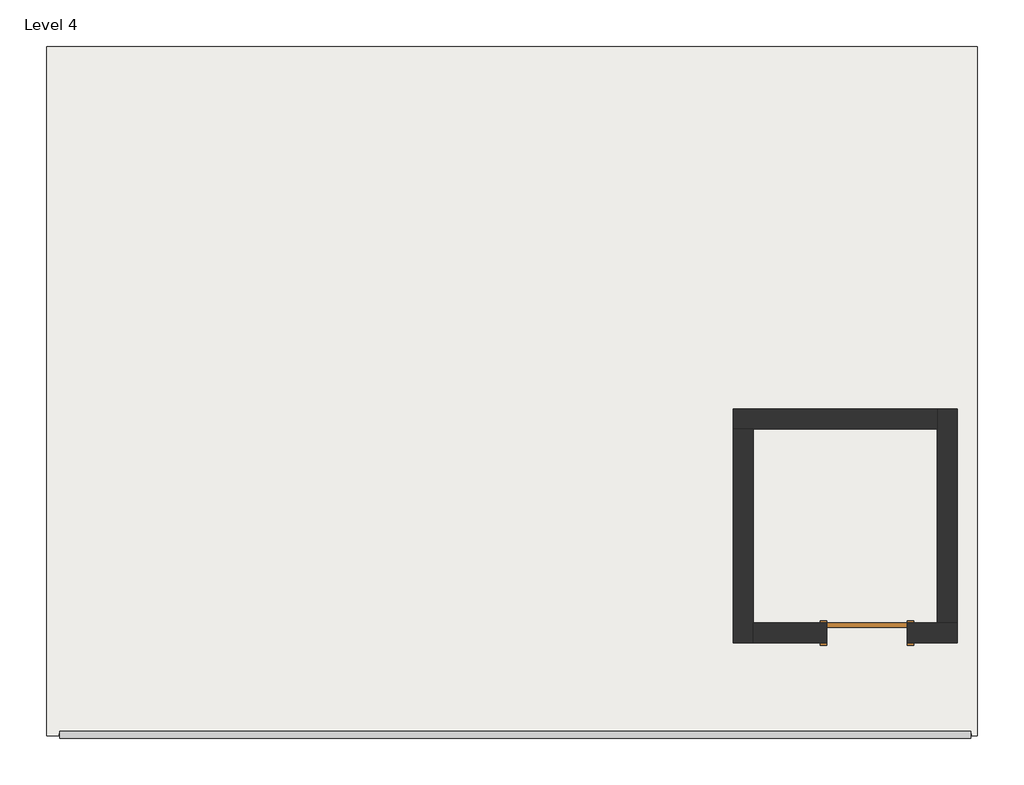
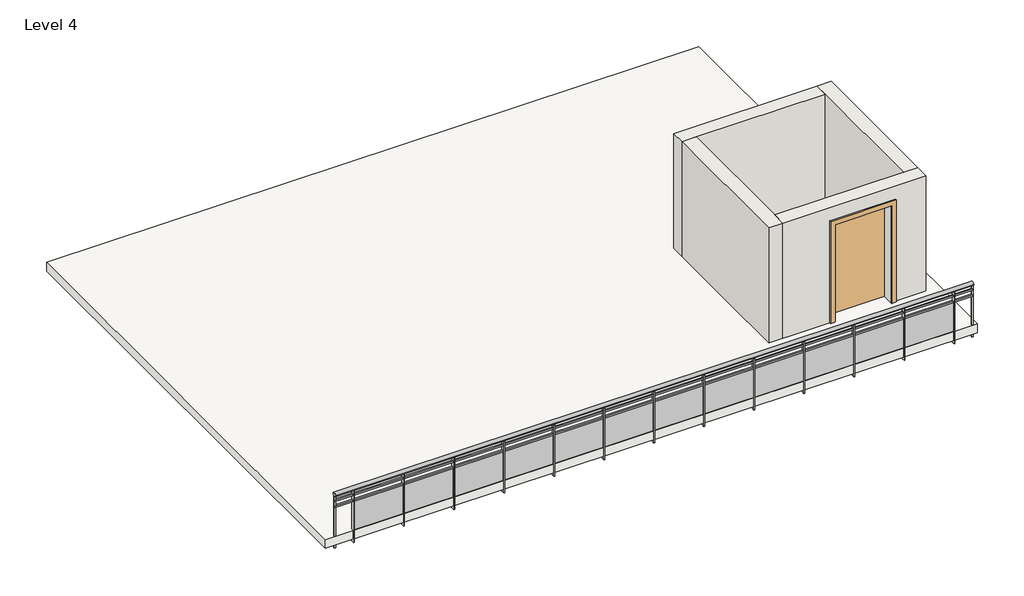
# One storey: 4 walls, 1 door, 1 railing, 1 roof.
"""IFC4 building model written with IfcOpenShell, lengths in millimetres."""

from ifc_helpers import new_model, si_unit, point, frame, origin, place, context, project, spatial, polyline, ellipse_curve, trimmed, outline, extrude, faceted_brep, transform, mapped, element, save
from ifc_brep_helpers import plane_surface, extruded_surface, advanced_brep
from components import door_0ca8825f

model = new_model("IFC4")

# Units and contexts
model_context = context("Model", 3, world=origin())
ifc_project = project(units=[si_unit("LENGTHUNIT", "METRE", prefix="MILLI")], contexts=[model_context])

# Site, building, storey
site = spatial("IfcSite", under=ifc_project)
building = spatial("IfcBuilding", under=site)
storey = spatial("IfcBuildingStorey", under=building, Name="Level 4", Elevation=6248.4)

# Door
placement = place(None, origin())
door_shape = door_0ca8825f(model_context)
element("IfcDoor", 1, ObjectType="Single-Flush : 36\" x 84\"", at=placement, inside=storey, context=model_context, shape_type="MappedRepresentation", body=[
    mapped(door_shape, transform((-524.0379854, -4635.5538577, 6248.4), x_axis=(1.0, 0.0, 0.0), y_axis=(0.0, 1.0, 0.0), z_axis=(0.0, 0.0, 1.0))),
])

# Railing
element("IfcRailing", 2, ObjectType="Glass Panel - Bottom Fill", at=placement, inside=storey, context=model_context, shape_type="SolidModel", body=[
    advanced_brep(
    [(657.0620146, -5831.8506821, 7416.8), (657.0620146, -5755.6506821, 7416.8), (-9706.1379854, -5831.8506821, 7416.8), (-9706.1379854, -5755.6506821, 7416.8)],
    [
        (0, 1, ellipse_curve(frame((657.0620146, -5793.7506821, 7416.8), z_axis=(1.0, 0.0, 0.0), x_axis=(0.0, 1.0, 0.0)), 38.1, 28.575)),
        (1, 0, ellipse_curve(frame((657.0620146, -5793.7506821, 7416.8), z_axis=(1.0, 0.0, 0.0), x_axis=(0.0, 1.0, 0.0)), 38.1, 28.575)),
        (2, 3, ellipse_curve(frame((-9706.1379854, -5793.7506821, 7416.8), z_axis=(-1.0, 0.0, 0.0), x_axis=(0.0, 1.0, 0.0)), 38.1, 28.575)),
        (3, 2, ellipse_curve(frame((-9706.1379854, -5793.7506821, 7416.8), z_axis=(-1.0, 0.0, 0.0), x_axis=(0.0, 1.0, 0.0)), 38.1, 28.575)),
        (0, 2),
        (3, 1),
    ],
    [
        plane_surface(frame((657.0620146, -5793.7506821, 7416.8), z_axis=(1.0, 0.0, 0.0), x_axis=(0.0, -1.0, 0.0))),
        plane_surface(frame((-9706.1379854, -5793.7506821, 7416.8), z_axis=(-1.0, 0.0, 0.0), x_axis=(0.0, -1.0, 0.0))),
        extruded_surface(trimmed(ellipse_curve(frame((-9706.1379854, -5793.7506821, 7416.8), z_axis=(1.0, 0.0, 0.0), x_axis=(0.0, 1.0, 0.0)), 38.1, 28.575), [point((-9706.1379854, -5831.8506821, 7416.8))], [point((-9706.1379854, -5755.6506821, 7416.8))], True, "CARTESIAN"), (10363.2, 0.0, 0.0), 10363.2),
        extruded_surface(trimmed(ellipse_curve(frame((-9706.1379854, -5793.7506821, 7416.8), z_axis=(1.0, 0.0, 0.0), x_axis=(0.0, 1.0, 0.0)), 38.1, 28.575), [point((-9706.1379854, -5755.6506821, 7416.8))], [point((-9706.1379854, -5831.8506821, 7416.8))], True, "CARTESIAN"), (10363.2, 0.0, 0.0), 10363.2),
    ],
    [
        (0, [[1, 2]]),
        (1, [[3, 4]]),
        (2, [[-1, 5, -4, 6]]),
        (3, [[-2, -6, -3, -5]]),
    ],
),
    extrude(outline(polyline([(657.0620146, -5781.0506821), (657.0620146, -5806.4506821), (-9706.1379854, -5806.4506821), (-9706.1379854, -5781.0506821), (657.0620146, -5781.0506821)])), frame((0.0, 0.0, 7302.5), z_axis=(0.0, 0.0, 1.0), x_axis=(1.0, 0.0, 0.0)), (0.0, 0.0, 1.0), 25.4),
    extrude(outline(polyline([(657.0620146, -5781.0506821), (657.0620146, -5806.4506821), (-9706.1379854, -5806.4506821), (-9706.1379854, -5781.0506821), (657.0620146, -5781.0506821)])), frame((0.0, 0.0, 7200.9), z_axis=(0.0, 0.0, 1.0), x_axis=(1.0, 0.0, 0.0)), (0.0, 0.0, 1.0), 25.4),
    extrude(outline(polyline([(-9394.9879854, -5768.3506821), (-9394.9879854, -5819.1506821), (-9407.6879854, -5819.1506821), (-9407.6879854, -5768.3506821), (-9394.9879854, -5768.3506821)])), frame((0.0, 0.0, 6502.4), z_axis=(0.0, 0.0, 1.0), x_axis=(1.0, 0.0, 0.0)), (0.0, 0.0, 1.0), 885.825),
    extrude(outline(polyline([(-8588.5379854, -5800.2858391), (-9401.3379854, -5800.2858391), (-9401.3379854, -5793.9358391), (-8588.5379854, -5793.9358391), (-8588.5379854, -5800.2858391)])), frame((0.0, 0.0, 6604.0), z_axis=(0.0, 0.0, 1.0), x_axis=(1.0, 0.0, 0.0)), (0.0, 0.0, 1.0), 596.9),
    extrude(outline(polyline([(-8582.1879854, -5768.3506821), (-8582.1879854, -5819.1506821), (-8594.8879854, -5819.1506821), (-8594.8879854, -5768.3506821), (-8582.1879854, -5768.3506821)])), frame((0.0, 0.0, 6502.4), z_axis=(0.0, 0.0, 1.0), x_axis=(1.0, 0.0, 0.0)), (0.0, 0.0, 1.0), 885.825),
    extrude(outline(polyline([(-7775.7379854, -5800.2858391), (-8588.5379854, -5800.2858391), (-8588.5379854, -5793.9358391), (-7775.7379854, -5793.9358391), (-7775.7379854, -5800.2858391)])), frame((0.0, 0.0, 6604.0), z_axis=(0.0, 0.0, 1.0), x_axis=(1.0, 0.0, 0.0)), (0.0, 0.0, 1.0), 596.9),
    extrude(outline(polyline([(-7769.3879854, -5768.3506821), (-7769.3879854, -5819.1506821), (-7782.0879854, -5819.1506821), (-7782.0879854, -5768.3506821), (-7769.3879854, -5768.3506821)])), frame((0.0, 0.0, 6502.4), z_axis=(0.0, 0.0, 1.0), x_axis=(1.0, 0.0, 0.0)), (0.0, 0.0, 1.0), 885.825),
    extrude(outline(polyline([(-6962.9379854, -5800.2858391), (-7775.7379854, -5800.2858391), (-7775.7379854, -5793.9358391), (-6962.9379854, -5793.9358391), (-6962.9379854, -5800.2858391)])), frame((0.0, 0.0, 6604.0), z_axis=(0.0, 0.0, 1.0), x_axis=(1.0, 0.0, 0.0)), (0.0, 0.0, 1.0), 596.9),
    extrude(outline(polyline([(-6956.5879854, -5768.3506821), (-6956.5879854, -5819.1506821), (-6969.2879854, -5819.1506821), (-6969.2879854, -5768.3506821), (-6956.5879854, -5768.3506821)])), frame((0.0, 0.0, 6502.4), z_axis=(0.0, 0.0, 1.0), x_axis=(1.0, 0.0, 0.0)), (0.0, 0.0, 1.0), 885.825),
    extrude(outline(polyline([(-6150.1379854, -5800.2858391), (-6962.9379854, -5800.2858391), (-6962.9379854, -5793.9358391), (-6150.1379854, -5793.9358391), (-6150.1379854, -5800.2858391)])), frame((0.0, 0.0, 6604.0), z_axis=(0.0, 0.0, 1.0), x_axis=(1.0, 0.0, 0.0)), (0.0, 0.0, 1.0), 596.9),
    extrude(outline(polyline([(-6143.7879854, -5768.3506821), (-6143.7879854, -5819.1506821), (-6156.4879854, -5819.1506821), (-6156.4879854, -5768.3506821), (-6143.7879854, -5768.3506821)])), frame((0.0, 0.0, 6502.4), z_axis=(0.0, 0.0, 1.0), x_axis=(1.0, 0.0, 0.0)), (0.0, 0.0, 1.0), 885.825),
    extrude(outline(polyline([(-5337.3379854, -5800.2858391), (-6150.1379854, -5800.2858391), (-6150.1379854, -5793.9358391), (-5337.3379854, -5793.9358391), (-5337.3379854, -5800.2858391)])), frame((0.0, 0.0, 6604.0), z_axis=(0.0, 0.0, 1.0), x_axis=(1.0, 0.0, 0.0)), (0.0, 0.0, 1.0), 596.9),
    extrude(outline(polyline([(-5330.9879854, -5768.3506821), (-5330.9879854, -5819.1506821), (-5343.6879854, -5819.1506821), (-5343.6879854, -5768.3506821), (-5330.9879854, -5768.3506821)])), frame((0.0, 0.0, 6502.4), z_axis=(0.0, 0.0, 1.0), x_axis=(1.0, 0.0, 0.0)), (0.0, 0.0, 1.0), 885.825),
    extrude(outline(polyline([(-4524.5379854, -5800.2858391), (-5337.3379854, -5800.2858391), (-5337.3379854, -5793.9358391), (-4524.5379854, -5793.9358391), (-4524.5379854, -5800.2858391)])), frame((0.0, 0.0, 6604.0), z_axis=(0.0, 0.0, 1.0), x_axis=(1.0, 0.0, 0.0)), (0.0, 0.0, 1.0), 596.9),
    extrude(outline(polyline([(-4518.1879854, -5768.3506821), (-4518.1879854, -5819.1506821), (-4530.8879854, -5819.1506821), (-4530.8879854, -5768.3506821), (-4518.1879854, -5768.3506821)])), frame((0.0, 0.0, 6502.4), z_axis=(0.0, 0.0, 1.0), x_axis=(1.0, 0.0, 0.0)), (0.0, 0.0, 1.0), 885.825),
    extrude(outline(polyline([(-3711.7379854, -5800.2858391), (-4524.5379854, -5800.2858391), (-4524.5379854, -5793.9358391), (-3711.7379854, -5793.9358391), (-3711.7379854, -5800.2858391)])), frame((0.0, 0.0, 6604.0), z_axis=(0.0, 0.0, 1.0), x_axis=(1.0, 0.0, 0.0)), (0.0, 0.0, 1.0), 596.9),
    extrude(outline(polyline([(-3705.3879854, -5768.3506821), (-3705.3879854, -5819.1506821), (-3718.0879854, -5819.1506821), (-3718.0879854, -5768.3506821), (-3705.3879854, -5768.3506821)])), frame((0.0, 0.0, 6502.4), z_axis=(0.0, 0.0, 1.0), x_axis=(1.0, 0.0, 0.0)), (0.0, 0.0, 1.0), 885.825),
    extrude(outline(polyline([(-2898.9379854, -5800.2858391), (-3711.7379854, -5800.2858391), (-3711.7379854, -5793.9358391), (-2898.9379854, -5793.9358391), (-2898.9379854, -5800.2858391)])), frame((0.0, 0.0, 6604.0), z_axis=(0.0, 0.0, 1.0), x_axis=(1.0, 0.0, 0.0)), (0.0, 0.0, 1.0), 596.9),
    extrude(outline(polyline([(-2892.5879854, -5768.3506821), (-2892.5879854, -5819.1506821), (-2905.2879854, -5819.1506821), (-2905.2879854, -5768.3506821), (-2892.5879854, -5768.3506821)])), frame((0.0, 0.0, 6502.4), z_axis=(0.0, 0.0, 1.0), x_axis=(1.0, 0.0, 0.0)), (0.0, 0.0, 1.0), 885.825),
    extrude(outline(polyline([(-2086.1379854, -5800.2858391), (-2898.9379854, -5800.2858391), (-2898.9379854, -5793.9358391), (-2086.1379854, -5793.9358391), (-2086.1379854, -5800.2858391)])), frame((0.0, 0.0, 6604.0), z_axis=(0.0, 0.0, 1.0), x_axis=(1.0, 0.0, 0.0)), (0.0, 0.0, 1.0), 596.9),
    extrude(outline(polyline([(-2079.7879854, -5768.3506821), (-2079.7879854, -5819.1506821), (-2092.4879854, -5819.1506821), (-2092.4879854, -5768.3506821), (-2079.7879854, -5768.3506821)])), frame((0.0, 0.0, 6502.4), z_axis=(0.0, 0.0, 1.0), x_axis=(1.0, 0.0, 0.0)), (0.0, 0.0, 1.0), 885.825),
    extrude(outline(polyline([(-1273.3379854, -5800.2858391), (-2086.1379854, -5800.2858391), (-2086.1379854, -5793.9358391), (-1273.3379854, -5793.9358391), (-1273.3379854, -5800.2858391)])), frame((0.0, 0.0, 6604.0), z_axis=(0.0, 0.0, 1.0), x_axis=(1.0, 0.0, 0.0)), (0.0, 0.0, 1.0), 596.9),
    extrude(outline(polyline([(-1266.9879854, -5768.3506821), (-1266.9879854, -5819.1506821), (-1279.6879854, -5819.1506821), (-1279.6879854, -5768.3506821), (-1266.9879854, -5768.3506821)])), frame((0.0, 0.0, 6502.4), z_axis=(0.0, 0.0, 1.0), x_axis=(1.0, 0.0, 0.0)), (0.0, 0.0, 1.0), 885.825),
    extrude(outline(polyline([(-460.5379854, -5800.2858391), (-1273.3379854, -5800.2858391), (-1273.3379854, -5793.9358391), (-460.5379854, -5793.9358391), (-460.5379854, -5800.2858391)])), frame((0.0, 0.0, 6604.0), z_axis=(0.0, 0.0, 1.0), x_axis=(1.0, 0.0, 0.0)), (0.0, 0.0, 1.0), 596.9),
    extrude(outline(polyline([(-454.1879854, -5768.3506821), (-454.1879854, -5819.1506821), (-466.8879854, -5819.1506821), (-466.8879854, -5768.3506821), (-454.1879854, -5768.3506821)])), frame((0.0, 0.0, 6502.4), z_axis=(0.0, 0.0, 1.0), x_axis=(1.0, 0.0, 0.0)), (0.0, 0.0, 1.0), 885.825),
    extrude(outline(polyline([(352.2620146, -5800.2858391), (-460.5379854, -5800.2858391), (-460.5379854, -5793.9358391), (352.2620146, -5793.9358391), (352.2620146, -5800.2858391)])), frame((0.0, 0.0, 6604.0), z_axis=(0.0, 0.0, 1.0), x_axis=(1.0, 0.0, 0.0)), (0.0, 0.0, 1.0), 596.9),
    extrude(outline(polyline([(358.6120146, -5768.3506821), (358.6120146, -5819.1506821), (345.9120146, -5819.1506821), (345.9120146, -5768.3506821), (358.6120146, -5768.3506821)])), frame((0.0, 0.0, 6502.4), z_axis=(0.0, 0.0, 1.0), x_axis=(1.0, 0.0, 0.0)), (0.0, 0.0, 1.0), 885.825),
    extrude(outline(polyline([(-9693.4379854, -5784.2256821), (-9693.4379854, -5803.2756821), (-9712.4879854, -5803.2756821), (-9712.4879854, -5784.2256821), (-9693.4379854, -5784.2256821)])), frame((0.0, 0.0, 6502.4), z_axis=(0.0, 0.0, 1.0), x_axis=(1.0, 0.0, 0.0)), (0.0, 0.0, 1.0), 885.825),
    extrude(outline(polyline([(663.4120146, -5784.2256821), (663.4120146, -5803.2756821), (644.3620146, -5803.2756821), (644.3620146, -5784.2256821), (663.4120146, -5784.2256821)])), frame((0.0, 0.0, 6502.4), z_axis=(0.0, 0.0, 1.0), x_axis=(1.0, 0.0, 0.0)), (0.0, 0.0, 1.0), 885.825),
])

# Roof
element("IfcRoof", 3, ObjectType="6\" floor", at=placement, inside=storey, context=model_context, shape_type="SweptSolid", body=[
    extrude(outline(polyline([(733.2620146, -5806.4506821), (-9858.5379854, -5806.4506821), (-9858.5379854, 2042.1493179), (733.2620146, 2042.1493179), (733.2620146, -5806.4506821)])), frame((0.0, 0.0, 6553.2), z_axis=(0.0, 0.0, 1.0), x_axis=(1.0, 0.0, 0.0)), (0.0, 0.0, 1.0), 152.4),
])

# Walls
element("IfcWall", 4, ObjectType="9\" wall", at=placement, inside=storey, context=model_context, shape_type="Brep", body=[
    faceted_brep([(504.6620146, -4521.2538577, 6248.4), (276.0620146, -4521.2538577, 6248.4), (-66.8379854, -4521.2538577, 6248.4), (-66.8379854, -4521.2538577, 8382.0), (-981.2379854, -4521.2538577, 8382.0), (-981.2379854, -4521.2538577, 6248.4), (-1819.4379854, -4521.2538577, 6248.4), (-1819.4379854, -4521.2538577, 8686.8), (276.0620146, -4521.2538577, 8686.8), (504.6620146, -4521.2538577, 8686.8), (-66.8379854, -4749.8538577, 8382.0), (-66.8379854, -4749.8538577, 6248.4), (504.6620146, -4749.8538577, 6248.4), (504.6620146, -4749.8538577, 8686.8), (-1819.4379854, -4749.8538577, 8686.8), (-1819.4379854, -4749.8538577, 6248.4), (-981.2379854, -4749.8538577, 6248.4), (-981.2379854, -4749.8538577, 8382.0)], [[[0, 1, 2, 3, 4, 5, 6, 7, 8, 9]], [[10, 11, 12, 13, 14, 15, 16, 17]], [[16, 15, 6, 5]], [[12, 11, 2, 1, 0]], [[9, 8, 7, 14, 13]], [[0, 9, 13, 12]], [[7, 6, 15, 14]], [[3, 2, 11, 10]], [[4, 3, 10, 17]], [[5, 4, 17, 16]]]),
])
element("IfcWall", 5, ObjectType="9\" wall", at=placement, inside=storey, context=model_context, shape_type="Brep", body=[
    faceted_brep([(276.0620146, -2082.8538577, 6248.4), (276.0620146, -2311.4538577, 6248.4), (276.0620146, -4521.2538577, 6248.4), (276.0620146, -4521.2538577, 8686.8), (276.0620146, -2311.4538577, 8686.8), (276.0620146, -2082.8538577, 8686.8), (504.6620146, -2082.8538577, 6248.4), (504.6620146, -2082.8538577, 8686.8), (504.6620146, -4521.2538577, 8686.8), (504.6620146, -4521.2538577, 6248.4)], [[[0, 1, 2, 3, 4, 5]], [[6, 7, 8, 9]], [[2, 1, 0, 6, 9]], [[5, 4, 3, 8, 7]], [[0, 5, 7, 6]], [[3, 2, 9, 8]]]),
])
element("IfcWall", 6, ObjectType="9\" wall", at=placement, inside=storey, context=model_context, shape_type="Brep", body=[
    faceted_brep([(-2048.0379854, -2311.4538577, 6248.4), (-1819.4379854, -2311.4538577, 6248.4), (276.0620146, -2311.4538577, 6248.4), (276.0620146, -2311.4538577, 8686.8), (-1819.4379854, -2311.4538577, 8686.8), (-2048.0379854, -2311.4538577, 8686.8), (-2048.0379854, -2082.8538577, 6248.4), (-2048.0379854, -2082.8538577, 8686.8), (276.0620146, -2082.8538577, 8686.8), (276.0620146, -2082.8538577, 6248.4)], [[[0, 1, 2, 3, 4, 5]], [[6, 7, 8, 9]], [[2, 1, 0, 6, 9]], [[5, 4, 3, 8, 7]], [[0, 5, 7, 6]], [[3, 2, 9, 8]]]),
])
element("IfcWall", 7, ObjectType="9\" wall", at=placement, inside=storey, context=model_context, shape_type="Brep", body=[
    faceted_brep([(-1819.4379854, -4749.8538577, 6248.4), (-1819.4379854, -4521.2538577, 6248.4), (-1819.4379854, -2311.4538577, 6248.4), (-1819.4379854, -2311.4538577, 8686.8), (-1819.4379854, -4521.2538577, 8686.8), (-1819.4379854, -4749.8538577, 8686.8), (-2048.0379854, -4749.8538577, 6248.4), (-2048.0379854, -4749.8538577, 8686.8), (-2048.0379854, -2311.4538577, 8686.8), (-2048.0379854, -2311.4538577, 6248.4)], [[[0, 1, 2, 3, 4, 5]], [[6, 7, 8, 9]], [[2, 1, 0, 6, 9]], [[5, 4, 3, 8, 7]], [[0, 5, 7, 6]], [[3, 2, 9, 8]]]),
])

save(model, "model.ifc")

# Revit data of these elements
# Type "Single-Flush : 36\" x 84\""
#   Type Mark = "1"
#   Construction Type Id = "MDOOR"
#   Assembly Code = "C1020"
#   Analytic Construction = "Metal"
#   Thickness = 0' - 2"
#   Heat Transfer Coefficient (U) = 0.651978 BTU/(h·ft²·°F)
#   Height = 7' - 0"
#   Trim Projection Ext = 0' - 1"
#   Trim Projection Int = 0' - 1"
#   Trim Width = 0' - 3"
#   Width = 3' - 0"
#   Define Thermal Properties by = 1
#   Define Thermal Properties by = 1
#   Door Material = door
#   Frame Material = door
#   Visual Light Transmittance = 0
#   Solar Heat Gain Coefficient = 0
#   Function = (empty or 0)
#   Wall Closure = (empty or 0)
# Type "Glass Panel - Bottom Fill"
#   Assembly Code = "C2010400"
#   built-in parameter 1008612 = 0.0416667 (stored number, unit not read)
#   built-in parameter 1008611 = 0.0416667 (stored number, unit not read)
#   built-in parameter 1008609 = 0.333333 (stored number, unit not read)
#   built-in parameter 1008604 = 0.166667 (stored number, unit not read)
#   built-in parameter 1008603 = 0.166667 (stored number, unit not read)
#   Railing Height = 3' - 0"
#   built-in parameter 1008630 = 2
#   built-in parameter 1008610 = 2
#   built-in parameter 1008618 = Baluster - Square : 3/4"
# Type "6\" floor"
#   Assembly Code = "B1020"
#   Layers, outside or top first: 0' - 6" no material (function 1)
# Type "9\" wall"
#   Assembly Code = "B2010"
# Element 1 (IfcDoor, "Single-Flush : 36\" x 84\"")
#   Phase Created = New Construction
#   Materials on its faces: "door"
# Element 2 (IfcRailing, "Glass Panel - Bottom Fill")
#   built-in parameter 1008621 = 0.833333 (stored number, unit not read)
#   Phase Created = New Construction
#   Materials on its faces: "Glass"
# Element 3 (IfcRoof, "6\" floor")
#   built-in parameter 1001705 = 22 (stored number, unit not read)
#   built-in parameter 1001701 = 1 (stored number, unit not read)
#   built-in parameter 1001710 = 33615
#   Phase Created = New Construction
#   Materials on its faces: "Default Roof"
# Elements 4, 5, 6, 7 (IfcWall, "9\" wall")
#   Top Offset = 0' - 0"
#   Base Offset = 0' - 0"
#   wall height = 8' - 0"
#   Phase Created = New Construction
#   Base Constraint = Level 4
#   Top Constraint = Level 5
# Materials
#   "door": class "Generic", colour RGB 120 120 120, transparency 0, Cost = 0
#   "Glass": class "Glass", colour RGB 0 128 192, transparency 0.75, Description = "Soda Lime Glass", Cost = 0
#   "Default Roof": colour RGB 88 101 114, transparency 0, Cost = 0
